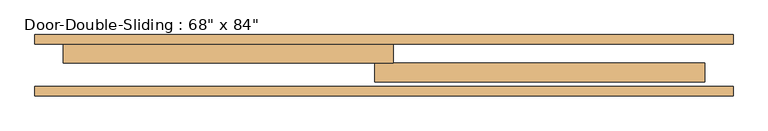
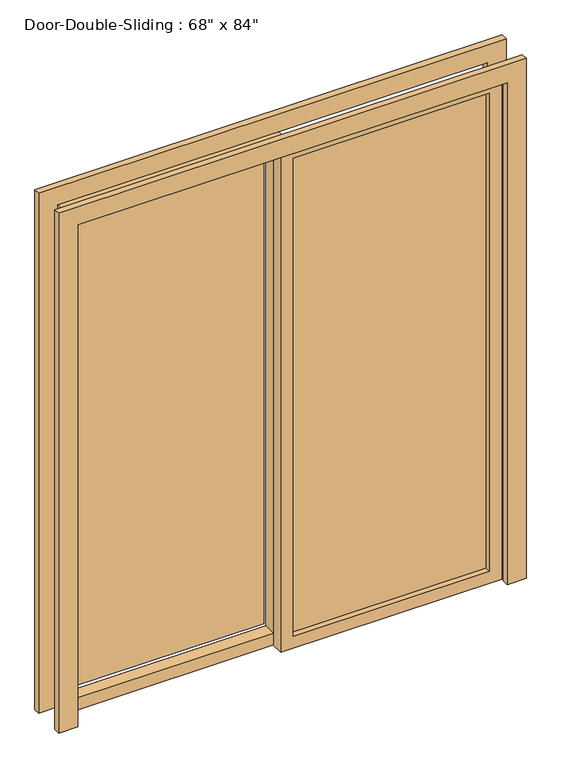
"""IFC4 building model written with IfcOpenShell, lengths in millimetres: door geometry."""

from ifc_helpers import new_model, si_unit, frame, origin, place, context, project, spatial, polyline, outline, extrude, source, transform, mapped, element, save


def door_505787c2(model_context):
    return source(origin(), model_context, "Body", "SweptSolid", [
        extrude(outline(polyline([(0.0, 939.8), (2209.8, 939.8), (2209.8, -939.8), (0.0, -939.8), (0.0, -863.6), (2133.6, -863.6), (2133.6, 863.6), (0.0, 863.6), (0.0, 939.8)])), frame((0.0, 184.15, 0.0), z_axis=(0.0, 1.0, 0.0), x_axis=(0.0, 0.0, 1.0)), (0.0, 0.0, 1.0), 25.4),
        extrude(outline(polyline([(0.0, -939.8), (0.0, -863.6), (2133.6, -863.6), (2133.6, 863.6), (0.0, 863.6), (0.0, 939.8), (2209.8, 939.8), (2209.8, -939.8), (0.0, -939.8)])), frame((0.0, 44.45, 0.0), z_axis=(0.0, 1.0, 0.0), x_axis=(0.0, 0.0, 1.0)), (0.0, 0.0, 1.0), 25.4),
        extrude(outline(polyline([(2133.6, 25.4), (2133.6, -863.6), (0.0, -863.6), (0.0, 25.4), (2133.6, 25.4)]), holes=[polyline([(2082.8, -25.4), (50.8, -25.4), (50.8, -812.8), (2082.8, -812.8), (2082.8, -25.4)])]), frame((0.0, 133.35, 0.0), z_axis=(0.0, 1.0, 0.0), x_axis=(0.0, 0.0, 1.0)), (0.0, 0.0, 1.0), 50.8),
        extrude(outline(polyline([(2133.6, -25.4), (0.0, -25.4), (0.0, 863.6), (2133.6, 863.6), (2133.6, -25.4)]), holes=[polyline([(2082.8, 25.4), (2082.8, 812.8), (50.8, 812.8), (50.8, 25.4), (2082.8, 25.4)])]), frame((0.0, 82.55, 0.0), z_axis=(0.0, 1.0, 0.0), x_axis=(0.0, 0.0, 1.0)), (0.0, 0.0, 1.0), 50.8),
        extrude(outline(polyline([(-25.4, 200.025), (-812.8, 200.025), (-812.8, 206.375), (-25.4, 206.375), (-25.4, 200.025)])), frame((0.0, 0.0, 50.8), z_axis=(0.0, 0.0, 1.0), x_axis=(1.0, 0.0, 0.0)), (0.0, 0.0, 1.0), 2032.0),
        extrude(outline(polyline([(25.4, 111.125), (812.8, 111.125), (812.8, 104.775), (25.4, 104.775), (25.4, 111.125)])), frame((0.0, 0.0, 50.8), z_axis=(0.0, 0.0, 1.0), x_axis=(1.0, 0.0, 0.0)), (0.0, 0.0, 1.0), 2032.0),
    ])


if __name__ == "__main__":
    model = new_model("IFC4")
    model_context = context("Model", 3, world=origin())
    ifc_project = project(units=[si_unit("LENGTHUNIT", "METRE", prefix="MILLI")], contexts=[model_context])
    site = spatial("IfcSite", under=ifc_project)
    building = spatial("IfcBuilding", under=site)
    placement = place(None, origin())
    door_shape = door_505787c2(model_context)
    element("IfcDoor", 1, ObjectType="Door-Double-Sliding : 68\" x 84\"", at=placement, inside=building, context=model_context, shape_type="MappedRepresentation", body=[
        mapped(door_shape, transform((0.0, 0.0, 0.0), x_axis=(1.0, 0.0, 0.0), y_axis=(0.0, 1.0, 0.0), z_axis=(0.0, 0.0, 1.0))),
    ])
    save(model, "model.ifc")

# Revit data of these elements
# Type "Door-Double-Sliding : 68\" x 84\""
#   Type Mark = "12"
#   Construction Type Id = "opn-d45"
#   Assembly Code = "C1020"
#   Analytic Construction = "Wood frame, double glass door "
#   Thickness = 0' - 2"
#   Thermal Resistance (R) = 1.8150 (h·ft²·°F)/BTU
#   Heat Transfer Coefficient (U) = 0.5510 BTU/(h·ft²·°F)
#   Height = 7' - 0"
#   Rail Width = 0' - 2"
#   Stiles = 0' - 2"
#   Trim Projection Ext = 0' - 1"
#   Trim Projection Int = 0' - 1"
#   Trim Width = 0' - 3"
#   Width = 5' - 8"
#   Define Thermal Properties by = 1
#   Glazing = Glass
#   Panel Material = Wood - Birch - Solid Stained Light Low Gloss
#   Trim Material = Paint - Sienna
#   Visual Light Transmittance = 0
#   Solar Heat Gain Coefficient = 0
#   Function = (empty or 0)
#   Wall Closure = (empty or 0)
# Element 1 (IfcDoor, "Door-Double-Sliding : 68\" x 84\"")
#   Materials on its faces: "Paint - Sienna", "Wood - Birch - Solid Stained Light Low Gloss", "Glass"
# Materials
#   "Glass": class "Glass", colour RGB 0 128 192, transparency 0.75, Description = "Soda Lime Glass", Cost = 0
#   "Wood - Birch - Solid Stained Light Low Gloss": class "Wood", colour RGB 210 159 95, transparency 0, Cost = 0
#   "Paint - Sienna": colour RGB 118 70 51, transparency 0, Cost = 0
